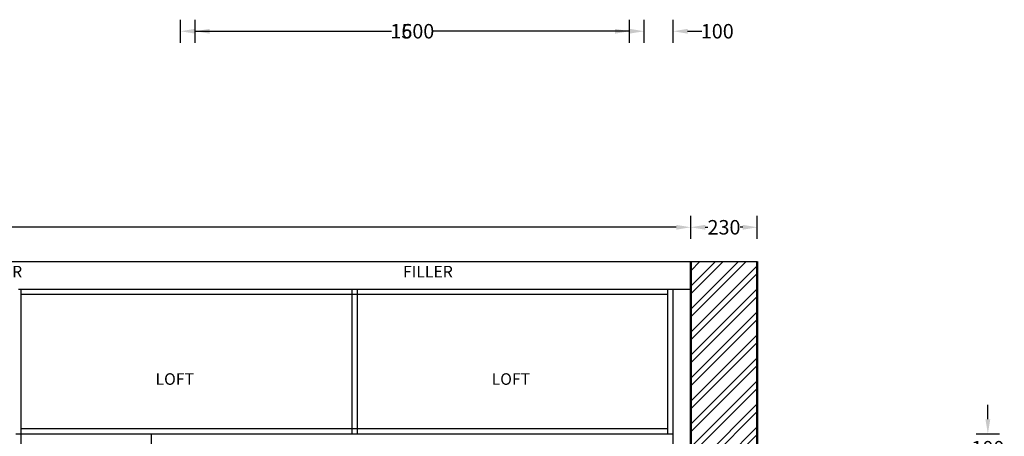
# Model space of a CAD drawing. Units: millimetres. Extents: x -472 to 16192, y -4730 to 4331.
# Tile 8 of 8: x 12774 to 16173, y -1895 to -455. Entities that reach past the tile are written whole.
import ezdxf

# ---------------------------------------------------------------- set-up
doc = ezdxf.new("R2010")
doc.units = ezdxf.units.MM
doc.header["$MEASUREMENT"] = 0
for name, color, linetype, lineweight in [('A-ANNO-DIMS', 2, 'Continuous', 18), ('A-ANNO-TEXT', 6, 'Continuous', 18), ('A-ELEV', 7, 'Continuous', 25), ('A-WALL', 7, 'Continuous', 50), ('A-WALL-PATT', 8, 'Continuous', 13)]:
    doc.layers.add(name, color=color, linetype=linetype, lineweight=lineweight)
doc.styles.get("Standard").update_dxf_attribs({"font": 'arial.ttf'})
doc.dimstyles.get("Standard").update_dxf_attribs({"dimtxt": 50, "dimasz": 50, "dimexe": 40, "dimexo": 40, "dimgap": 0.09, "dimtad": 0, "dimtih": 1, "dimtoh": 1, "dimdec": 0, "dimzin": 0, "dimdsep": 46, "dimtxsty": 'Standard', "dimcen": 0.09, "dimclrd": 1, "dimclre": 3, "dimclrt": 6, "dimadec": 0, "dimazin": 0, "dimtfac": 1, "dimtdec": 0, "dimtofl": 0, "dimtmove": 0, "dimatfit": 3, "dimfxl": 40, "dimfxlon": 1, "dimtolj": 1, "dimtzin": 0, "dimarcsym": 0})

# ---------------------------------------------------------------- blocks, each defined once
blk = doc.blocks.new('*D44')
at = {"layer": 'A-ANNO-DIMS', "color": 0, "lineweight": -2, "transparency": 16777216}
for p, q in [((9950.7, -1212.4), (9950.7, -1132.4)), ((15090.7, -1212.4), (15090.7, -1132.4)), ((10000.7, -1172.4), (12446, -1172.4)), ((15040.7, -1172.4), (12595.3, -1172.4))]:
    blk.add_line(p, q, dxfattribs=at)
at = {"layer": 'A-ANNO-DIMS', "color": 0, "transparency": 16777216}
for points in [[(10000.7, -1164.1), (10000.7, -1180.8), (9950.7, -1172.4)], [(15040.7, -1164.1), (15040.7, -1180.8), (15090.7, -1172.4)]]:
    blk.add_solid(points, dxfattribs=at)
at = {"layer": 'Defpoints', "color": 0, "transparency": 16777216}
for p in [(15090.7, -1172.4), (9950.7, -1290.9), (15090.7, -1290.9)]:
    blk.add_point(p, dxfattribs=at)
at = {"layer": 'A-ANNO-DIMS', "color": 0, "transparency": 16777216, "insert": (12520.7, -1172.4), "char_height": 50, "attachment_point": 5}
blk.add_mtext('\\A1;5140', dxfattribs=at)
blk = doc.blocks.new('*D45')
at = {"layer": 'A-ANNO-DIMS', "color": 0, "lineweight": -2, "transparency": 16777216}
for p, q in [((15090.7, -1212.4), (15090.7, -1132.4)), ((15320.7, -1212.4), (15320.7, -1132.4)), ((15140.7, -1172.4), (15150, -1172.4)), ((15270.7, -1172.4), (15261.3, -1172.4))]:
    blk.add_line(p, q, dxfattribs=at)
at = {"layer": 'A-ANNO-DIMS', "color": 0, "transparency": 16777216}
for points in [[(15140.7, -1164.1), (15140.7, -1180.8), (15090.7, -1172.4)], [(15270.7, -1164.1), (15270.7, -1180.8), (15320.7, -1172.4)]]:
    blk.add_solid(points, dxfattribs=at)
at = {"layer": 'Defpoints', "color": 0, "transparency": 16777216}
for p in [(15320.7, -1172.4), (15090.7, -1290.9), (15320.7, -1290.9)]:
    blk.add_point(p, dxfattribs=at)
at = {"layer": 'A-ANNO-DIMS', "color": 0, "transparency": 16777216, "insert": (15205.7, -1172.4), "char_height": 50, "attachment_point": 5}
blk.add_mtext('\\A1;230', dxfattribs=at)
blk = doc.blocks.new('*D100')
at = {"layer": 'A-ANNO-DIMS', "color": 1, "lineweight": -2, "transparency": 16777216}
for p, q in [((16116.7, -1835.9), (16116.7, -1785.9)), ((16116.7, -2035.9), (16116.7, -2085.9))]:
    blk.add_line(p, q, dxfattribs=at)
at = {"layer": 'A-ANNO-DIMS', "color": 3, "lineweight": -2, "transparency": 16777216}
for p, q in [((16076.7, -1885.9), (16156.7, -1885.9)), ((16076.7, -1985.9), (16156.7, -1985.9))]:
    blk.add_line(p, q, dxfattribs=at)
at = {"layer": 'A-ANNO-DIMS', "color": 1, "transparency": 16777216}
for points in [[(16108.3, -1835.9), (16125, -1835.9), (16116.7, -1885.9)], [(16108.3, -2035.9), (16125, -2035.9), (16116.7, -1985.9)]]:
    blk.add_solid(points, dxfattribs=at)
at = {"layer": 'Defpoints', "color": 0, "transparency": 16777216}
for p in [(5309, -1885.9), (5209, -1985.9), (16116.7, -1985.9)]:
    blk.add_point(p, dxfattribs=at)
at = {"layer": 'A-ANNO-DIMS', "color": 6, "transparency": 16777216, "insert": (16116.7, -1935.9), "char_height": 50, "attachment_point": 5}
blk.add_mtext('\\A1;100', dxfattribs=at)
blk = doc.blocks.new('*D105')
at = {"layer": 'A-ANNO-DIMS', "color": 3, "lineweight": -2, "transparency": 16777216}
for p, q in [((14929.7, -534.9), (14929.7, -454.9)), ((15029.7, -534.9), (15029.7, -454.9))]:
    blk.add_line(p, q, dxfattribs=at)
at = {"layer": 'A-ANNO-DIMS', "color": 1, "lineweight": -2, "transparency": 16777216}
for p, q in [((14879.7, -494.9), (14829.7, -494.9)), ((15079.7, -494.9), (15129.7, -494.9))]:
    blk.add_line(p, q, dxfattribs=at)
at = {"layer": 'A-ANNO-DIMS', "color": 1, "transparency": 16777216}
for points in [[(14879.7, -486.6), (14879.7, -503.2), (14929.7, -494.9)], [(15079.7, -486.6), (15079.7, -503.2), (15029.7, -494.9)]]:
    blk.add_solid(points, dxfattribs=at)
at = {"layer": 'Defpoints', "color": 0, "transparency": 16777216}
for p in [(15029.7, -494.9), (15029.7, -1885.9), (14929.7, -1985.9)]:
    blk.add_point(p, dxfattribs=at)
at = {"layer": 'A-ANNO-DIMS', "color": 6, "transparency": 16777216, "insert": (15182.5, -494.9), "char_height": 50, "attachment_point": 5}
blk.add_mtext('\\A1;100', dxfattribs=at)
blk = doc.blocks.new('*D106')
at = {"layer": 'A-ANNO-DIMS', "color": 3, "lineweight": -2, "transparency": 16777216}
for p, q in [((13329.7, -534.9), (13329.7, -454.9)), ((14929.7, -534.9), (14929.7, -454.9))]:
    blk.add_line(p, q, dxfattribs=at)
at = {"layer": 'A-ANNO-DIMS', "color": 1, "lineweight": -2, "transparency": 16777216}
for p, q in [((13379.7, -494.9), (14057.3, -494.9)), ((14879.7, -494.9), (14202, -494.9))]:
    blk.add_line(p, q, dxfattribs=at)
at = {"layer": 'A-ANNO-DIMS', "color": 1, "transparency": 16777216}
for points in [[(13379.7, -486.6), (13379.7, -503.2), (13329.7, -494.9)], [(14879.7, -486.6), (14879.7, -503.2), (14929.7, -494.9)]]:
    blk.add_solid(points, dxfattribs=at)
at = {"layer": 'Defpoints', "color": 0, "transparency": 16777216}
for p in [(14929.7, -494.9), (13329.7, -1985.9), (14929.7, -1985.9)]:
    blk.add_point(p, dxfattribs=at)
at = {"layer": 'A-ANNO-DIMS', "color": 6, "transparency": 16777216, "insert": (14129.7, -494.9), "char_height": 50, "attachment_point": 5}
blk.add_mtext('\\A1;1600', dxfattribs=at)
blk = doc.blocks.new('*D107')
at = {"layer": 'A-ANNO-DIMS', "color": 3, "lineweight": -2, "transparency": 16777216}
for p, q in [((13379.7, -534.9), (13379.7, -454.9)), ((14879.7, -534.9), (14879.7, -454.9))]:
    blk.add_line(p, q, dxfattribs=at)
at = {"layer": 'A-ANNO-DIMS', "color": 1, "lineweight": -2, "transparency": 16777216}
for p, q in [((13429.7, -494.9), (14057.3, -494.9)), ((14829.7, -494.9), (14202, -494.9))]:
    blk.add_line(p, q, dxfattribs=at)
at = {"layer": 'A-ANNO-DIMS', "color": 1, "transparency": 16777216}
for points in [[(13429.7, -486.6), (13429.7, -503.2), (13379.7, -494.9)], [(14829.7, -486.6), (14829.7, -503.2), (14879.7, -494.9)]]:
    blk.add_solid(points, dxfattribs=at)
at = {"layer": 'Defpoints', "color": 0, "transparency": 16777216}
for p in [(14879.7, -494.9), (13379.7, -2035.9), (14879.7, -2035.9)]:
    blk.add_point(p, dxfattribs=at)
at = {"layer": 'A-ANNO-DIMS', "color": 6, "transparency": 16777216, "insert": (14129.7, -494.9), "char_height": 50, "attachment_point": 5}
blk.add_mtext('\\A1;1500', dxfattribs=at)
blk = doc.blocks.new('*D108')
at = {"layer": 'A-ANNO-DIMS', "color": 1, "lineweight": -2, "transparency": 16777216}
for p, q in [((16116.7, -1835.9), (16116.7, -1785.9)), ((16116.7, -2035.9), (16116.7, -2085.9))]:
    blk.add_line(p, q, dxfattribs=at)
at = {"layer": 'A-ANNO-DIMS', "color": 3, "lineweight": -2, "transparency": 16777216}
for p, q in [((16076.7, -1885.9), (16156.7, -1885.9)), ((16076.7, -1985.9), (16156.7, -1985.9))]:
    blk.add_line(p, q, dxfattribs=at)
at = {"layer": 'A-ANNO-DIMS', "color": 1, "transparency": 16777216}
for points in [[(16108.3, -1835.9), (16125, -1835.9), (16116.7, -1885.9)], [(16108.3, -2035.9), (16125, -2035.9), (16116.7, -1985.9)]]:
    blk.add_solid(points, dxfattribs=at)
at = {"layer": 'Defpoints', "color": 0, "transparency": 16777216}
for p in [(15029.7, -1885.9), (14929.7, -1985.9), (16116.7, -1985.9)]:
    blk.add_point(p, dxfattribs=at)
at = {"layer": 'A-ANNO-DIMS', "color": 6, "transparency": 16777216, "insert": (16116.7, -1935.9), "char_height": 50, "attachment_point": 5}
blk.add_mtext('\\A1;100', dxfattribs=at)

msp = doc.modelspace()

# ---------------------------------------------------------------- hatches: boundary and pattern name
at = {"layer": 'A-WALL-PATT'}
h = msp.add_hatch(dxfattribs=at)
h.set_pattern_fill('ANSI32', color=256, scale=150)
h.paths.add_polyline_path([(9720.7, -1290.9), (9720.7, -4285.9), (9950.7, -4285.9), (9950.7, -4185.9), (9950.7, -1885.9), (9950.7, -1290.9)])
h.paths.add_polyline_path([(5370, -4285.9), (5600, -4285.9), (5600, -1290.9), (5370, -1290.9)])
h.paths.add_polyline_path([(15320.7, -1290.9), (15090.7, -1290.9), (15090.7, -4285.9), (15320.7, -4285.9)])
h.paths.add_polyline_path([(0, -4285.9), (230, -4285.9), (230, -4185.9), (230, -1885.9), (230, -1290.9), (0, -1290.9)])

# ---------------------------------------------------------------- linework, layer by layer
at = {"layer": 'A-ELEV'}
for p, q in [((9720.7, -1290.9), (15320.7, -1290.9)), ((12769.7, -1385.9), (15090.7, -1385.9)), ((12778.7, -1885.9), (12778.7, -1385.9)), ((13921.2, -1385.9), (13921.2, -1885.9)), ((13939.2, -1385.9), (13939.2, -1885.9)), ((15011.7, -1885.9), (15011.7, -1385.9)), ((15029.7, -1885.9), (15029.7, -1385.9)), ((12778.7, -1403.9), (15011.7, -1403.9)), ((12778.7, -1867.9), (15011.7, -1867.9)), ((12760.7, -1885.9), (15029.7, -1885.9)), ((12778.7, -4185.9), (12778.7, -1885.9)), ((13229.7, -3685.9), (13229.7, -1885.9)), ((15029.7, -3635.9), (15029.7, -1885.9))]:
    msp.add_line(p, q, dxfattribs=at)
at = {"layer": 'A-WALL'}
for p, q in [((15090.7, -4285.9), (15090.7, -1290.9)), ((15320.7, -4285.9), (15320.7, -1290.9))]:
    msp.add_line(p, q, dxfattribs=at)

# ---------------------------------------------------------------- texts
at = {"layer": 'A-ANNO-TEXT', "char_height": 40, "attachment_point": 1}
for s, insert in [('FILLER', (12610.5, -1305.7)), ('FILLER', (14097.3, -1305.7)), ('LOFT', (13243, -1676.9)), ('LOFT', (14403.5, -1676.9))]:
    msp.add_mtext_dynamic_manual_height_columns(s, width=327.678, gutter_width=1, heights=[0], dxfattribs=dict(at, insert=insert))

# ---------------------------------------------------------------- dimensions: what is measured, and where the dimension line sits
at = {"layer": 'A-ANNO-DIMS'}
for base, p1, p2, override, picture, middle in [((14929.7, -494.9), (13329.7, -1985.9), (14929.7, -1985.9), {"dimdec": 0, "dimlfac": 1, "dimrnd": 0, "dimzin": 0, "dimdsep": 46, "dimlunit": 2}, '*D106', (14129.7, -494.9)), ((14879.7, -494.9), (13379.7, -2035.9), (14879.7, -2035.9), {"dimdec": 0, "dimlfac": 1, "dimrnd": 0, "dimzin": 0, "dimdsep": 46, "dimlunit": 2}, '*D107', (14129.7, -494.9)), ((15029.7, -494.9), (14929.7, -1985.9), (15029.7, -1885.9), {"dimdec": 0, "dimlfac": 1, "dimrnd": 0, "dimzin": 0, "dimdsep": 46, "dimlunit": 2}, '*D105', (15182.5, -494.9)), ((15090.7, -1172.4), (9950.7, -1290.9), (15090.7, -1290.9), {"dimclrd": 0, "dimclre": 0, "dimclrt": 0}, '*D44', (12520.7, -1172.4)), ((15320.7, -1172.4), (15090.7, -1290.9), (15320.7, -1290.9), {"dimclrd": 0, "dimclre": 0, "dimclrt": 0}, '*D45', (15205.7, -1172.4))]:
    dim = msp.add_linear_dim(base=base, p1=p1, p2=p2, dimstyle='Standard', override=override, dxfattribs=at)
    dim.commit()
    dim.dimension.update_dxf_attribs({"geometry": picture, "text_midpoint": middle})
for p1, p2, picture in [((5309, -1885.9), (5209, -1985.9), '*D100'), ((15029.7, -1885.9), (14929.7, -1985.9), '*D108')]:
    dim = msp.add_linear_dim(base=(16116.7, -1985.9), p1=p1, p2=p2, angle=90, dimstyle='Standard', override={"dimdec": 0, "dimlfac": 1, "dimrnd": 0, "dimzin": 0, "dimdsep": 46, "dimlunit": 2}, dxfattribs=at)
    dim.commit()
    dim.dimension.update_dxf_attribs({"geometry": picture, "text_midpoint": (16116.7, -1935.9)})

doc.saveas('drawing.dxf')
